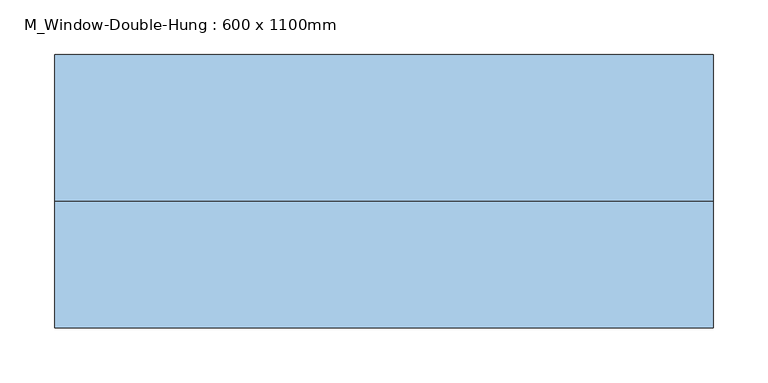
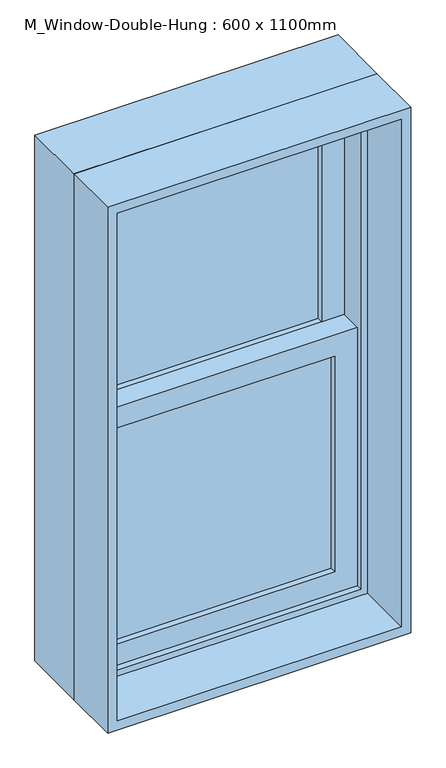
"""IFC4 building model written with IfcOpenShell, lengths in millimetres: window geometry, M_Window-Double-Hung : 600 x 1100mm."""

from ifc_helpers import new_model, si_unit, frame, origin, place, context, project, spatial, polyline, outline, extrude, source, transform, mapped, element, save


def m_window_double_hung_600_x_1100mm_c7e90a65(model_context):
    return source(origin(), model_context, "Body", "SweptSolid", [
        extrude(outline(polyline([(223.8, 45.15), (223.8, 38.8), (-223.8, 38.8), (-223.8, 45.15), (223.8, 45.15)])), frame((0.0, 0.0, 990.6), z_axis=(0.0, 0.0, 1.0), x_axis=(1.0, 0.0, 0.0)), (0.0, 0.0, 1.0), 451.575),
        extrude(outline(polyline([(-223.8, 32.45), (223.8, 32.45), (223.8, 26.1), (-223.8, 26.1), (-223.8, 32.45)])), frame((0.0, 0.0, 990.6), z_axis=(0.0, 0.0, 1.0), x_axis=(1.0, 0.0, 0.0)), (0.0, 0.0, 1.0), 451.575),
        extrude(outline(polyline([(223.8, 89.6), (223.8, 83.25), (-223.8, 83.25), (-223.8, 89.6), (223.8, 89.6)])), frame((0.0, 0.0, 1486.625), z_axis=(0.0, 0.0, 1.0), x_axis=(1.0, 0.0, 0.0)), (0.0, 0.0, 1.0), 451.575),
        extrude(outline(polyline([(-223.8, 76.9), (223.8, 76.9), (223.8, 70.55), (-223.8, 70.55), (-223.8, 76.9)])), frame((0.0, 0.0, 1486.625), z_axis=(0.0, 0.0, 1.0), x_axis=(1.0, 0.0, 0.0)), (0.0, 0.0, 1.0), 451.575),
        extrude(outline(polyline([(1486.625, -268.25), (946.15, -268.25), (946.15, 268.25), (1486.625, 268.25), (1486.625, -268.25)]), holes=[polyline([(1442.175, 223.8), (990.6, 223.8), (990.6, -223.8), (1442.175, -223.8), (1442.175, 223.8)])]), frame((0.0, 13.4, 0.0), z_axis=(0.0, 1.0, 0.0), x_axis=(0.0, 0.0, 1.0)), (0.0, 0.0, 1.0), 44.45),
        extrude(outline(polyline([(1982.65, -268.25), (1442.175, -268.25), (1442.175, 268.25), (1982.65, 268.25), (1982.65, -268.25)]), holes=[polyline([(1938.2, 223.8), (1486.625, 223.8), (1486.625, -223.8), (1938.2, -223.8), (1938.2, 223.8)])]), frame((0.0, 57.85, 0.0), z_axis=(0.0, 1.0, 0.0), x_axis=(0.0, 0.0, 1.0)), (0.0, 0.0, 1.0), 44.45),
        extrude(outline(polyline([(2014.4, -300.0), (914.4, -300.0), (914.4, 300.0), (2014.4, 300.0), (2014.4, -300.0)]), holes=[polyline([(1982.65, 268.25), (946.15, 268.25), (946.15, -268.25), (1982.65, -268.25), (1982.65, 268.25)])]), frame((0.0, 0.7, 0.0), z_axis=(0.0, 1.0, 0.0), x_axis=(0.0, 0.0, 1.0)), (0.0, 0.0, 1.0), 133.35),
        extrude(outline(polyline([(2014.4, 300.0), (2014.4, -300.0), (914.4, -300.0), (914.4, 300.0), (2014.4, 300.0)]), holes=[polyline([(1995.35, 280.95), (933.45, 280.95), (933.45, -280.95), (1995.35, -280.95), (1995.35, 280.95)])]), frame((0.0, -115.0, 0.0), z_axis=(0.0, 1.0, 0.0), x_axis=(0.0, 0.0, 1.0)), (0.0, 0.0, 1.0), 115.7),
    ])


if __name__ == "__main__":
    model = new_model("IFC4")
    model_context = context("Model", 3, world=origin())
    ifc_project = project(units=[si_unit("LENGTHUNIT", "METRE", prefix="MILLI")], contexts=[model_context])
    site = spatial("IfcSite", under=ifc_project)
    building = spatial("IfcBuilding", under=site)
    placement = place(None, origin())
    m_window_double_hung_600_x_1100mm_shape = m_window_double_hung_600_x_1100mm_c7e90a65(model_context)
    element("IfcWindow", 1, ObjectType="M_Window-Double-Hung : 600 x 1100mm", at=placement, inside=building, context=model_context, shape_type="MappedRepresentation", body=[
        mapped(m_window_double_hung_600_x_1100mm_shape, transform((0.0, 0.0, 0.0), x_axis=(1.0, 0.0, 0.0), y_axis=(0.0, 1.0, 0.0), z_axis=(0.0, 0.0, 1.0))),
    ])
    save(model, "model.ifc")

# Revit data of these elements
# Type "M_Window-Double-Hung : 600 x 1100mm"
#   Type Mark = "W1"
#   Fire Rating = "0.5h"
#   Construction Type Id = "DG-DR"
#   Assembly Code = "B2020100"
#   Analytic Construction = "Double glazing - domestic"
#   Wall Thickness [instance default] = 0.15 m
#   Window Inset [instance default] = 0 m
#   Visual Light Transmittance = 0.81
#   Thermal Resistance (R) = 0.319569 (m²·K)/W
#   Solar Heat Gain Coefficient = 0.76
#   Muntin Width = 0.4476 m
#   Muntin Height = 0.451575 m
#   Interior Wall Closure [instance default] = 0.0357 m
#   Rough Width = 0.615 m
#   Rough Height = 1.115 m
#   Frame Extension [instance default] = 0.03175 m
#   Exterior Wall Closure [instance default] = 0.0127 m
#   Extension Jamb [instance default] = 0.0357 m
#   Heat Transfer Coefficient (U) = 3.12929 W/(m²·K)
#   Height = 1.1 m
#   Width = 0.6 m
#   Define Thermal Properties by = 1
#   Top Muntin Visibility = yes
#   Indicator Visibility [instance default] = yes
#   Extension Jamb Visibility [instance default] = yes
#   Interior Trim Visibility [instance default] = yes
#   Exterior Trim Visibility [instance default] = yes
#   Define Thermal Properties by = 1
#   Bottom Muntin Visibility = yes
#   Muntin Pattern = M_Muntin Pattern_2x2 : M_Muntin Pattern_2x2
#   Interior Trim Material = Wood - Stained
#   Interior Trim = M_Trim-Window-Interior-Flat : Picture Frame
#   Exterior Trim Material = Clad - White
#   Exterior Trim = M_Trim-Window-Exterior-Flat : with Sill
#   Glass Panel Material = Glass
#   Exterior Frame Material = Clad - White
#   Interior Frame Material = Wood - Stained
#   Wall Closure = (empty or 0)
# Element 1 (IfcWindow, "M_Window-Double-Hung : 600 x 1100mm")
#   Wall Thickness = 0.23 m
#   Extension Jamb = 0.1157 m
#   Materials on its faces: "Wood - Stained", "Glass", "Clad - White"
# Materials
#   "Wood - Stained": class "Wood", colour RGB 224 178 126, transparency 0, Cost = 0
#   "Clad - White": class "Wood", colour RGB 242 242 238, transparency 0, Cost = 0
#   "Glass": class "Glass", colour RGB 0 128 192, transparency 0.9, Description = "Soda Lime Glass", Cost = 0
